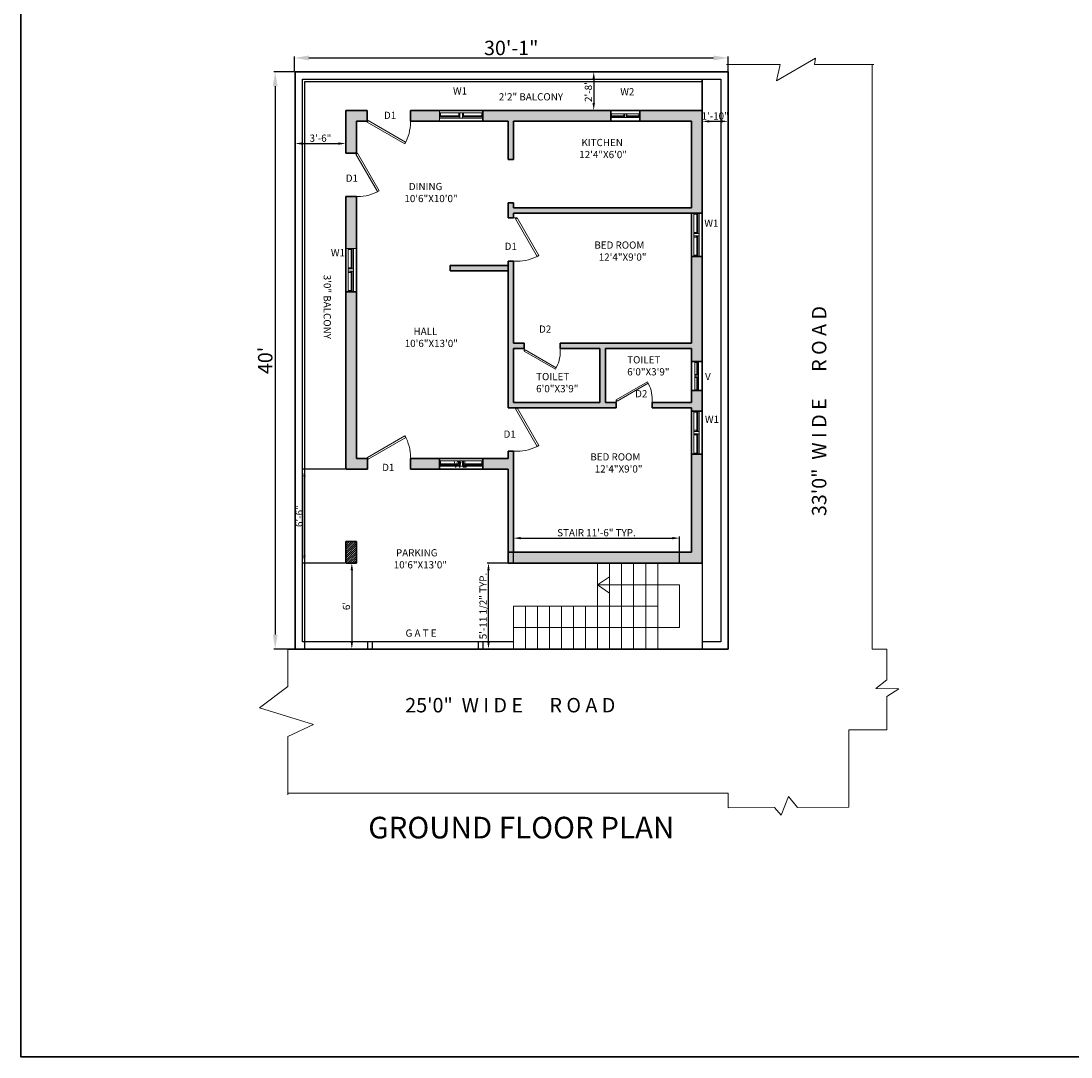
# Model space of a CAD drawing. Units: millimetres. Extents: x 50579 to 52843, y 62224 to 63803.
# Tile 1 of 5: x 50579 to 51453, y 62224 to 63086. Entities that reach past the tile are written whole.
import ezdxf

# ---------------------------------------------------------------- set-up
doc = ezdxf.new("R2010")
doc.units = ezdxf.units.MM
for name, color, linetype, lineweight in [('A-ANNO-DIMS', 2, 'Continuous', 18), ('A-ANNO-IDEN', 6, 'Continuous', 18), ('A-ANNO-TITL', 4, 'Continuous', 25), ('A-ANNO-TTLB', 7, 'Continuous', 35), ('A-AREA-IDEN', 6, 'Continuous', 18), ('A-COLS', 7, 'Continuous', 35), ('A-COLS-PATT', 8, 'Continuous', 13), ('A-FLOR-BALC', 7, 'Continuous', 25), ('A-FLOR-STRS', 7, 'Continuous', 18), ('A-GLAZ', 4, 'Continuous', 18), ('A-WALL', 7, 'Continuous', 35), ('A-WALL-PATT', 251, 'Continuous', 13), ('C-ANNO-TEXT', 4, 'Continuous', 18), ('C-PROP', 7, 'Continuous', 35), ('C-ROAD', 7, 'Continuous', 18), ('C-SITE-GATE', 7, 'Continuous', 25), ('C-SITE-WALL', 7, 'Continuous', 25), ('DOOR', 20, 'Continuous', 18)]:
    doc.layers.add(name, color=color, linetype=linetype, lineweight=lineweight)
doc.styles.get("Standard").update_dxf_attribs({"font": 'arial.ttf'})
doc.dimstyles.new('ISO-25', dxfattribs={"dimtxt": 6, "dimasz": 6, "dimexe": 1.25, "dimexo": 0.625, "dimtad": 1, "dimdec": 0, "dimlunit": 3, "dimtxsty": 'Standard', "dimcen": 2.5, "dimadec": 0, "dimazin": 0, "dimtfac": 1, "dimtdec": 0, "dimtmove": 0, "dimatfit": 3, "dimfxl": 1, "dimarcsym": 0})

# ---------------------------------------------------------------- blocks, each defined once
blk = doc.blocks.new('W1')
for p, q in [((50927.56, 62719.85), (50945.56, 62719.85)), ((50927.56, 62717.25), (50944.56, 62717.25)), ((50927.56, 62716.35), (50944.56, 62716.35)), ((50927.56, 62715.35), (50963.56, 62715.35)), ((50929.58, 62717.08), (50942.53, 62717.08)), ((50929.58, 62716.8), (50942.53, 62716.8)), ((50929.58, 62716.54), (50942.53, 62716.54)), ((50944.56, 62717.61), (50944.56, 62715.35)), ((50963.56, 62719.85), (50945.56, 62719.85)), ((50946.56, 62717.61), (50946.56, 62715.35)), ((50963.56, 62717.25), (50946.56, 62717.25)), ((50963.56, 62716.35), (50946.56, 62716.35)), ((50961.53, 62717.08), (50948.58, 62717.08)), ((50961.53, 62716.8), (50948.58, 62716.8)), ((50961.53, 62716.54), (50948.58, 62716.54))]:
    blk.add_line(p, q)
for points in [[(50927.56, 62712.85), (50927.56, 62721.85), (50963.56, 62721.85), (50963.56, 62712.85)], [(50927.56, 62719.85), (50928.5, 62719.85), (50928.5, 62717.61), (50927.56, 62717.61)], [(50928.59, 62717.25), (50929.58, 62717.25), (50929.58, 62716.35), (50928.59, 62716.35)], [(50943.52, 62717.25), (50942.53, 62717.25), (50942.53, 62716.35), (50943.52, 62716.35)], [(50944.56, 62719.85), (50943.61, 62719.85), (50943.61, 62717.61), (50944.56, 62717.61)], [(50946.56, 62719.85), (50947.5, 62719.85), (50947.5, 62717.61), (50946.56, 62717.61)], [(50947.59, 62717.25), (50948.58, 62717.25), (50948.58, 62716.35), (50947.59, 62716.35)], [(50962.52, 62717.25), (50961.53, 62717.25), (50961.53, 62716.35), (50962.52, 62716.35)], [(50963.56, 62719.85), (50962.61, 62719.85), (50962.61, 62717.61), (50963.56, 62717.61)]]:
    blk.add_lwpolyline(points, close=True)
blk = doc.blocks.new('*U3')
for p, q in [((0, 0), (0, -6)), ((40, 0), (40, -6))]:
    blk.add_line(p, q)
blk.add_lwpolyline([(0, 0), (34.64, 20), (35.52, 18.48), (0.87, -1.52)], close=True)
blk.add_arc((0, 0), 40, 0, 30)
blk = doc.blocks.new('*D5')
at = {"layer": 'A-ANNO-DIMS', "color": 0, "lineweight": -2, "transparency": 16777216}
for p, q in [((51052.14, 63043.35), (51057.07, 63043.35)), ((51055.82, 63037.35), (51055.82, 63017.35)), ((51052.14, 63011.35), (51057.07, 63011.35))]:
    blk.add_line(p, q, dxfattribs=at)
at = {"layer": 'A-ANNO-DIMS', "color": 0, "transparency": 16777216}
for points in [[(51054.82, 63037.35), (51056.82, 63037.35), (51055.82, 63043.35)], [(51054.82, 63017.35), (51056.82, 63017.35), (51055.82, 63011.35)]]:
    blk.add_solid(points, dxfattribs=at)
at = {"layer": 'Defpoints', "color": 0, "transparency": 16777216}
for p in [(51051.52, 63043.35), (51051.52, 63011.35), (51055.82, 63011.35)]:
    blk.add_point(p, dxfattribs=at)
at = {"layer": 'A-ANNO-DIMS', "color": 0, "transparency": 16777216, "insert": (51052.13, 63027.35), "char_height": 6, "attachment_point": 5, "rotation": 90}
blk.add_mtext('2\'-8"', dxfattribs=at)
blk = doc.blocks.new('*D6')
at = {"layer": 'A-ANNO-DIMS', "color": 0, "lineweight": -2, "transparency": 16777216}
for p, q in [((51146.02, 63010.73), (51146.02, 63000.95)), ((51167.52, 63010.73), (51167.52, 63000.95)), ((51161.52, 63002.2), (51152.02, 63002.2))]:
    blk.add_line(p, q, dxfattribs=at)
at = {"layer": 'A-ANNO-DIMS', "color": 0, "transparency": 16777216}
for points in [[(51152.02, 63003.2), (51152.02, 63001.2), (51146.02, 63002.2)], [(51161.52, 63003.2), (51161.52, 63001.2), (51167.52, 63002.2)]]:
    blk.add_solid(points, dxfattribs=at)
at = {"layer": 'Defpoints', "color": 0, "transparency": 16777216}
for p in [(51146.02, 63011.35), (51167.52, 63011.35), (51146.02, 63002.2)]:
    blk.add_point(p, dxfattribs=at)
at = {"layer": 'A-ANNO-DIMS', "color": 0, "transparency": 16777216, "insert": (51156.77, 63005.89), "char_height": 6, "attachment_point": 5}
blk.add_mtext('1\'-10"', dxfattribs=at)
blk = doc.blocks.new('*D7')
at = {"layer": 'A-ANNO-DIMS', "color": 0, "lineweight": -2, "transparency": 16777216}
for p, q in [((50807.52, 62977.26), (50807.52, 62984.99)), ((50813.52, 62983.74), (50843.52, 62983.74)), ((50849.52, 62977.26), (50849.52, 62984.99))]:
    blk.add_line(p, q, dxfattribs=at)
at = {"layer": 'A-ANNO-DIMS', "color": 0, "transparency": 16777216}
for points in [[(50813.52, 62984.74), (50813.52, 62982.74), (50807.52, 62983.74)], [(50843.52, 62984.74), (50843.52, 62982.74), (50849.52, 62983.74)]]:
    blk.add_solid(points, dxfattribs=at)
at = {"layer": 'Defpoints', "color": 0, "transparency": 16777216}
for p in [(50849.52, 62983.74), (50807.52, 62976.63), (50849.52, 62976.63)]:
    blk.add_point(p, dxfattribs=at)
at = {"layer": 'A-ANNO-DIMS', "color": 0, "transparency": 16777216, "insert": (50828.52, 62987.43), "char_height": 6, "attachment_point": 5}
blk.add_mtext('3\'-6"', dxfattribs=at)
blk = doc.blocks.new('*D8')
at = {"layer": 'A-ANNO-DIMS', "color": 0, "lineweight": -2, "transparency": 16777216}
for p, q in [((50806.89, 63043.35), (50789.64, 63043.35)), ((50790.89, 63031.35), (50790.89, 62575.35)), ((50806.89, 62563.35), (50789.64, 62563.35))]:
    blk.add_line(p, q, dxfattribs=at)
at = {"layer": 'A-ANNO-DIMS', "color": 0, "transparency": 16777216}
for points in [[(50788.89, 63031.35), (50792.89, 63031.35), (50790.89, 63043.35)], [(50788.89, 62575.35), (50792.89, 62575.35), (50790.89, 62563.35)]]:
    blk.add_solid(points, dxfattribs=at)
at = {"layer": 'Defpoints', "color": 0, "transparency": 16777216}
for p in [(50807.52, 63043.35), (50790.89, 62563.35), (50807.52, 62563.35)]:
    blk.add_point(p, dxfattribs=at)
at = {"layer": 'A-ANNO-DIMS', "color": 0, "transparency": 16777216, "insert": (50784.14, 62803.35), "char_height": 12, "attachment_point": 5, "rotation": 90}
blk.add_mtext("40'", dxfattribs=at)
blk = doc.blocks.new('*D9')
at = {"layer": 'A-ANNO-DIMS', "color": 0, "lineweight": -2, "transparency": 16777216}
for p, q in [((50806.89, 63043.98), (50806.89, 63056.19)), ((50818.89, 63054.94), (51155.52, 63054.94)), ((51167.52, 63043.98), (51167.52, 63056.19))]:
    blk.add_line(p, q, dxfattribs=at)
at = {"layer": 'A-ANNO-DIMS', "color": 0, "transparency": 16777216}
for points in [[(50818.89, 63056.94), (50818.89, 63052.94), (50806.89, 63054.94)], [(51155.52, 63056.94), (51155.52, 63052.94), (51167.52, 63054.94)]]:
    blk.add_solid(points, dxfattribs=at)
at = {"layer": 'Defpoints', "color": 0, "transparency": 16777216}
for p in [(51167.52, 63054.94), (50806.89, 63043.35), (51167.52, 63043.35)]:
    blk.add_point(p, dxfattribs=at)
at = {"layer": 'A-ANNO-DIMS', "color": 0, "transparency": 16777216, "insert": (50987.2, 63061.7), "char_height": 12, "attachment_point": 5}
blk.add_mtext('30\'-1"', dxfattribs=at)
blk = doc.blocks.new('*D10')
at = {"layer": 'A-ANNO-DIMS', "color": 0, "lineweight": -2, "transparency": 16777216}
for p, q in [((50854.64, 62634.85), (50855.88, 62634.85)), ((50854.63, 62628.85), (50854.63, 62569.35)), ((50854.64, 62563.35), (50855.88, 62563.35))]:
    blk.add_line(p, q, dxfattribs=at)
at = {"layer": 'A-ANNO-DIMS', "color": 0, "transparency": 16777216}
for points in [[(50853.63, 62628.85), (50855.63, 62628.85), (50854.63, 62634.85)], [(50853.63, 62569.35), (50855.63, 62569.35), (50854.63, 62563.35)]]:
    blk.add_solid(points, dxfattribs=at)
at = {"layer": 'Defpoints', "color": 0, "transparency": 16777216}
for p in [(50854.02, 62634.85), (50854.02, 62563.35), (50854.63, 62563.35)]:
    blk.add_point(p, dxfattribs=at)
at = {"layer": 'A-ANNO-DIMS', "color": 0, "transparency": 16777216, "insert": (50850.94, 62599.1), "char_height": 6, "attachment_point": 5, "rotation": 90}
blk.add_mtext("6'", dxfattribs=at)
blk = doc.blocks.new('WIN-W2-PLAN')
for p, q in [((0, 6.16), (12, 6.16)), ((0, 4.43), (11.33, 4.43)), ((0, 3.83), (11.33, 3.83)), ((0, 3.16), (24, 3.16)), ((1.35, 4.32), (9.98, 4.32)), ((1.35, 4.13), (9.98, 4.13)), ((1.35, 3.95), (9.98, 3.95)), ((11.33, 4.67), (11.33, 3.16)), ((24, 6.16), (12, 6.16)), ((12.67, 4.67), (12.67, 3.16)), ((24, 4.43), (12.67, 4.43)), ((24, 3.83), (12.67, 3.83)), ((22.65, 4.32), (14.02, 4.32)), ((22.65, 4.13), (14.02, 4.13)), ((22.65, 3.95), (14.02, 3.95))]:
    blk.add_line(p, q)
for points in [[(0, 0), (0, 9), (24, 9), (24, 0)], [(0, 6.16), (0.63, 6.16), (0.63, 4.67), (0, 4.67)], [(0.69, 4.43), (1.35, 4.43), (1.35, 3.83), (0.69, 3.83)], [(10.64, 4.43), (9.98, 4.43), (9.98, 3.83), (10.64, 3.83)], [(11.33, 6.16), (10.7, 6.16), (10.7, 4.67), (11.33, 4.67)], [(12.67, 6.16), (13.29, 6.16), (13.29, 4.67), (12.67, 4.67)], [(13.36, 4.43), (14.02, 4.43), (14.02, 3.83), (13.36, 3.83)], [(23.31, 4.43), (22.65, 4.43), (22.65, 3.83), (23.31, 3.83)], [(24, 6.16), (23.37, 6.16), (23.37, 4.67), (24, 4.67)]]:
    blk.add_lwpolyline(points, close=True)
blk = doc.blocks.new('VENT-V-PLAN')
for p, q in [((2.84, 24), (2.84, 12)), ((4.57, 24), (4.57, 12.67)), ((4.68, 22.65), (4.68, 14.02)), ((4.87, 22.65), (4.87, 14.02)), ((5.05, 22.65), (5.05, 14.02)), ((5.17, 24), (5.17, 12.67)), ((5.84, 24), (5.84, 0)), ((2.84, 0), (2.84, 12)), ((4.33, 12.67), (5.84, 12.67)), ((4.33, 11.33), (5.84, 11.33)), ((4.57, 0), (4.57, 11.33)), ((4.68, 1.35), (4.68, 9.98)), ((4.87, 1.35), (4.87, 9.98)), ((5.05, 1.35), (5.05, 9.98)), ((5.17, 0), (5.17, 11.33))]:
    blk.add_line(p, q)
for points in [[(9, 24), (0, 24), (0, 0), (9, 0)], [(2.84, 24), (2.84, 23.37), (4.33, 23.37), (4.33, 24)], [(4.57, 23.31), (4.57, 22.65), (5.17, 22.65), (5.17, 23.31)], [(2.84, 12.67), (2.84, 13.3), (4.33, 13.3), (4.33, 12.67)], [(2.84, 11.33), (2.84, 10.71), (4.33, 10.71), (4.33, 11.33)], [(4.57, 13.36), (4.57, 14.02), (5.17, 14.02), (5.17, 13.36)], [(4.57, 10.64), (4.57, 9.98), (5.17, 9.98), (5.17, 10.64)], [(2.84, 0), (2.84, 0.63), (4.33, 0.63), (4.33, 0)], [(4.57, 0.69), (4.57, 1.35), (5.17, 1.35), (5.17, 0.69)]]:
    blk.add_lwpolyline(points, close=True)
blk = doc.blocks.new('STAIR-RETURN-PLAN')
for p, q in [((70, 0), (70, 71.5)), ((80, 0), (80, 71.5)), ((90, 0), (90, 71.5)), ((100, 0), (100, 71.5)), ((110, 0), (110, 71.5)), ((120, 0), (120, 71.5)), ((70, 53.25), (80, 59.99)), ((138.14, 53.25), (70, 53.25)), ((70, 53.25), (80, 46.5)), ((138.14, 17.87), (138.14, 53.25)), ((0, 0), (0, 35.75)), ((120, 35.75), (0, 35.75)), ((10, 0), (10, 35.75)), ((20, 0), (20, 35.75)), ((30, 0), (30, 35.75)), ((40, 0), (40, 35.75)), ((50, 0), (50, 35.75)), ((60, 0), (60, 35.75)), ((0, 17.87), (138.14, 17.87))]:
    blk.add_line(p, q)
blk = doc.blocks.new('GATE-POST-PAIR')
for p, q in [((0, 6), (0, 0)), ((4, 6), (4, 0)), ((92.04, 6), (92.04, 0)), ((96.04, 6), (96.04, 0))]:
    blk.add_line(p, q)
blk = doc.blocks.new('*D33')
at = {"layer": 'A-ANNO-DIMS', "color": 0, "lineweight": -2, "transparency": 16777216}
for p, q in [((50989.02, 62635.48), (50989.02, 62656.82)), ((50995.02, 62655.57), (51121.16, 62655.57)), ((51127.16, 62635.48), (51127.16, 62656.82))]:
    blk.add_line(p, q, dxfattribs=at)
at = {"layer": 'A-ANNO-DIMS', "color": 0, "transparency": 16777216}
for points in [[(50995.02, 62656.57), (50995.02, 62654.57), (50989.02, 62655.57)], [(51121.16, 62656.57), (51121.16, 62654.57), (51127.16, 62655.57)]]:
    blk.add_solid(points, dxfattribs=at)
at = {"layer": 'Defpoints', "color": 0, "transparency": 16777216}
for p in [(51127.16, 62655.57), (50989.02, 62634.85), (51127.16, 62634.85)]:
    blk.add_point(p, dxfattribs=at)
at = {"layer": 'A-ANNO-DIMS', "color": 0, "transparency": 16777216, "insert": (51058.09, 62659.3), "char_height": 6, "attachment_point": 5}
blk.add_mtext('STAIR 11\'-6" TYP.', dxfattribs=at)
blk = doc.blocks.new('*D34')
at = {"layer": 'A-ANNO-DIMS', "color": 0, "lineweight": -2, "transparency": 16777216}
for p, q in [((50988.39, 62634.85), (50967.05, 62634.85)), ((50968.3, 62569.35), (50968.3, 62628.85)), ((50988.39, 62563.35), (50967.05, 62563.35))]:
    blk.add_line(p, q, dxfattribs=at)
at = {"layer": 'A-ANNO-DIMS', "color": 0, "transparency": 16777216}
for points in [[(50967.3, 62628.85), (50969.3, 62628.85), (50968.3, 62634.85)], [(50967.3, 62569.35), (50969.3, 62569.35), (50968.3, 62563.35)]]:
    blk.add_solid(points, dxfattribs=at)
at = {"layer": 'Defpoints', "color": 0, "transparency": 16777216}
for p in [(50968.3, 62634.85), (50989.02, 62634.85), (50989.02, 62563.35)]:
    blk.add_point(p, dxfattribs=at)
at = {"layer": 'A-ANNO-DIMS', "color": 0, "transparency": 16777216, "insert": (50964.57, 62599.1), "char_height": 6, "attachment_point": 5, "rotation": 90}
blk.add_mtext('5\'-11 1/2" TYP.', dxfattribs=at)
blk = doc.blocks.new('*D76')
at = {"layer": 'A-ANNO-DIMS', "color": 0, "lineweight": -2, "transparency": 16777216}
for p, q in [((50848.89, 62712.85), (50813.97, 62712.85)), ((50815.22, 62640.85), (50815.22, 62706.85)), ((50848.89, 62634.85), (50813.97, 62634.85))]:
    blk.add_line(p, q, dxfattribs=at)
at = {"layer": 'A-ANNO-DIMS', "color": 0, "transparency": 16777216}
for points in [[(50814.22, 62706.85), (50816.22, 62706.85), (50815.22, 62712.85)], [(50814.22, 62640.85), (50816.22, 62640.85), (50815.22, 62634.85)]]:
    blk.add_solid(points, dxfattribs=at)
at = {"layer": 'Defpoints', "color": 0, "transparency": 16777216}
for p in [(50815.22, 62712.85), (50849.52, 62712.85), (50849.52, 62634.85)]:
    blk.add_point(p, dxfattribs=at)
at = {"layer": 'A-ANNO-DIMS', "color": 0, "transparency": 16777216, "insert": (50811.53, 62673.85), "char_height": 6, "attachment_point": 5, "rotation": 90}
blk.add_mtext('6\'-6"', dxfattribs=at)

msp = doc.modelspace()

# ---------------------------------------------------------------- hatches: boundary and pattern name
at = {"layer": 'A-COLS-PATT'}
h = msp.add_hatch(dxfattribs=at)
h.set_pattern_fill('ANSI31', color=256, scale=0.4)
h.paths.add_polyline_path([(50858.52, 62643.85), (50858.52, 62652.85), (50849.52, 62652.85), (50849.52, 62634.85), (50858.52, 62634.85)])
at = {"layer": 'A-WALL-PATT'}
h = msp.add_hatch(color=256, dxfattribs=at)
h.dxf.hatch_style = 1
h.paths.add_polyline_path([(50858.52, 63002.35), (50867.4, 63002.35), (50867.4, 63006.85), (50867.4, 63011.35), (50849.52, 63011.35), (50849.52, 62975.7), (50858.52, 62975.7)])
h = msp.add_hatch(color=256, dxfattribs=at)
h.dxf.hatch_style = 1
h.paths.add_polyline_path([(50927.56, 63011.35), (50903.4, 63011.35), (50903.4, 63002.35), (50927.56, 63002.35)])
h = msp.add_hatch(color=256, dxfattribs=at)
h.dxf.hatch_style = 1
h.paths.add_polyline_path([(51070.05, 63011.35), (50963.56, 63011.35), (50963.56, 63002.35), (50984.52, 63002.35), (50984.52, 62970.35), (50989.02, 62970.35), (50989.02, 63002.35), (51070.05, 63002.35)])
h = msp.add_hatch(color=256, dxfattribs=at)
h.dxf.hatch_style = 1
h.paths.add_polyline_path([(51146.02, 63011.35), (51094.05, 63011.35), (51094.05, 63002.35), (51137.02, 63002.35), (51137.02, 62930.35), (50989.02, 62930.35), (50989.02, 62934.35), (50984.52, 62934.35), (50984.52, 62921.85), (50989.02, 62921.85), (50989.02, 62925.85), (51146.02, 62925.85)])
h = msp.add_hatch(color=256, dxfattribs=at)
h.dxf.hatch_style = 1
h.paths.add_polyline_path([(50858.52, 62939.7), (50854.02, 62939.7), (50849.52, 62939.7), (50849.52, 62896.5), (50858.52, 62896.5)])
h = msp.add_hatch(color=256, dxfattribs=at)
h.dxf.hatch_style = 1
h.paths.add_polyline_path([(51074.52, 62768.35), (51065.52, 62768.35), (51065.52, 62813.35), (51137.02, 62813.35), (51137.02, 62802.37), (51146.02, 62802.37), (51146.02, 62889.85), (51137.02, 62889.85), (51137.02, 62817.85), (51028.02, 62817.85), (51028.02, 62813.35), (51061.02, 62813.35), (51061.02, 62768.35), (50989.02, 62768.35), (50989.02, 62813.35), (50998.02, 62813.35), (50998.02, 62817.85), (50989.02, 62817.85), (50989.02, 62885.85), (50984.52, 62885.85), (50984.52, 62763.85), (51074.52, 62763.85)])
h = msp.add_hatch(color=256, dxfattribs=at)
h.dxf.hatch_style = 1
h.paths.add_polyline_path([(50984.52, 62882.35), (50936.52, 62882.35), (50936.52, 62877.85), (50984.52, 62877.85)])
h = msp.add_hatch(color=256, dxfattribs=at)
h.dxf.hatch_style = 1
h.paths.add_polyline_path([(50858.52, 62860.5), (50849.52, 62860.5), (50849.52, 62712.85), (50867.52, 62712.85), (50867.52, 62721.85), (50858.52, 62721.85)])
h = msp.add_hatch(color=256, dxfattribs=at)
h.dxf.hatch_style = 1
h.paths.add_polyline_path([(51146.02, 62778.37), (51137.02, 62778.37), (51137.02, 62768.35), (51104.52, 62768.35), (51104.52, 62766.1), (51104.52, 62763.85), (51137.02, 62763.85), (51137.02, 62761.3), (51146.02, 62761.3)])
h = msp.add_hatch(color=256, dxfattribs=at)
h.dxf.hatch_style = 1
h.paths.add_polyline_path([(50927.56, 62721.85), (50903.52, 62721.85), (50903.52, 62717.35), (50903.52, 62712.85), (50927.56, 62712.85)])
h = msp.add_hatch(color=256, dxfattribs=at)
h.dxf.hatch_style = 1
h.paths.add_polyline_path([(50989.02, 62727.85), (50984.52, 62727.85), (50984.52, 62721.85), (50963.56, 62721.85), (50963.56, 62712.85), (50984.52, 62712.85), (50984.52, 62643.85), (50989.02, 62643.85)])
h = msp.add_hatch(color=256, dxfattribs=at)
h.dxf.hatch_style = 1
h.paths.add_polyline_path([(51146.02, 62725.3), (51137.02, 62725.3), (51137.02, 62643.85), (50984.52, 62643.85), (50984.52, 62634.85), (51146.02, 62634.85)])

# ---------------------------------------------------------------- linework, layer by layer
at = {"layer": 'A-ANNO-TTLB'}
msp.add_lwpolyline([(50579.46, 63802.65), (52843.1, 63802.65), (52843.1, 62224.04), (50579.46, 62224.04)], close=True, dxfattribs=at)
at = {"layer": 'A-COLS'}
for p, q in [((50849.52, 62634.85), (50849.52, 62652.85)), ((50849.52, 62652.85), (50858.52, 62652.85)), ((50858.52, 62643.85), (50858.52, 62652.85)), ((50858.52, 62643.85), (50858.52, 62634.85)), ((50849.52, 62634.85), (50858.52, 62634.85))]:
    msp.add_line(p, q, dxfattribs=at)
at = {"layer": 'A-FLOR-BALC'}
for p, q in [((50815.52, 63035.35), (51146.02, 63035.35)), ((50815.52, 62563.35), (50815.52, 63035.35)), ((51146.02, 62634.85), (51146.02, 62563.35))]:
    msp.add_line(p, q, dxfattribs=at)
at = {"layer": 'A-WALL'}
for p, q in [((51146.02, 62634.85), (51146.02, 63037.35)), ((50849.52, 63011.35), (50867.4, 63011.35)), ((50849.52, 62975.7), (50849.52, 63011.35)), ((50867.4, 63002.35), (50867.4, 63011.35)), ((50903.4, 63002.35), (50903.4, 63011.35)), ((50903.4, 63011.35), (51146.02, 63011.35)), ((50963.56, 63011.35), (50963.56, 63002.35)), ((51070.05, 63011.35), (51070.05, 63002.35)), ((51094.05, 63011.35), (51094.05, 63002.35)), ((50858.52, 63002.35), (50867.4, 63002.35)), ((50858.52, 62975.7), (50858.52, 63002.35)), ((50903.4, 63002.35), (50984.52, 63002.35)), ((50984.52, 62970.35), (50984.52, 63002.35)), ((50989.02, 63002.35), (51137.02, 63002.35)), ((50989.02, 62970.35), (50989.02, 63002.35)), ((51137.02, 62930.35), (51137.02, 63002.35)), ((50849.52, 62975.7), (50858.52, 62975.7)), ((50984.52, 62970.35), (50989.02, 62970.35)), ((50849.52, 62939.7), (50858.52, 62939.7)), ((50849.52, 62712.85), (50849.52, 62939.7)), ((50858.52, 62877.85), (50858.52, 62939.7)), ((50984.52, 62934.35), (50989.02, 62934.35)), ((50984.52, 62921.85), (50984.52, 62934.35)), ((50989.02, 62930.35), (50989.02, 62934.35)), ((50989.02, 62930.35), (51137.02, 62930.35)), ((50984.52, 62921.85), (50989.02, 62921.85)), ((50989.02, 62925.85), (51146.02, 62925.85)), ((50989.02, 62921.85), (50989.02, 62925.85)), ((51137.02, 62817.85), (51137.02, 62925.85)), ((51137.02, 62889.85), (51146.02, 62889.85)), ((50858.52, 62721.85), (50858.52, 62877.85)), ((50936.52, 62882.35), (50984.52, 62882.35)), ((50936.52, 62877.85), (50936.52, 62882.35)), ((50936.52, 62877.85), (50984.52, 62877.85)), ((50984.52, 62885.85), (50989.02, 62885.85)), ((50984.52, 62763.85), (50984.52, 62885.85)), ((50989.02, 62817.85), (50989.02, 62885.85)), ((50849.52, 62860.5), (50858.52, 62860.5)), ((50989.02, 62817.85), (50998.02, 62817.85)), ((50998.02, 62813.35), (50998.02, 62817.85)), ((51028.02, 62813.35), (51028.02, 62817.85)), ((51028.02, 62817.85), (51137.02, 62817.85)), ((50989.02, 62813.35), (50998.02, 62813.35)), ((50989.02, 62768.35), (50989.02, 62813.35)), ((51028.02, 62813.35), (51061.02, 62813.35)), ((51061.02, 62768.35), (51061.02, 62813.35)), ((51065.52, 62768.35), (51065.52, 62813.35)), ((51065.52, 62813.35), (51137.02, 62813.35)), ((51137.02, 62768.35), (51137.02, 62813.35)), ((51137.02, 62802.37), (51146.02, 62802.37)), ((51137.02, 62778.37), (51146.02, 62778.37)), ((50984.52, 62763.85), (51074.52, 62763.85)), ((50989.02, 62768.35), (51061.02, 62768.35)), ((51065.52, 62768.35), (51074.52, 62768.35)), ((51074.52, 62768.35), (51074.52, 62763.85)), ((51104.52, 62768.35), (51104.52, 62763.85)), ((51104.52, 62768.35), (51137.02, 62768.35)), ((51104.52, 62763.85), (51137.02, 62763.85)), ((51137.02, 62643.85), (51137.02, 62763.85)), ((51137.02, 62761.3), (51146.02, 62761.3)), ((51137.02, 62761.3), (51146.02, 62761.3)), ((50858.52, 62721.85), (50867.52, 62721.85)), ((50867.52, 62721.85), (50867.52, 62712.85)), ((50903.52, 62721.85), (50903.52, 62712.85)), ((50903.52, 62721.85), (50984.52, 62721.85)), ((50927.56, 62721.85), (50927.56, 62712.85)), ((50963.56, 62721.85), (50963.56, 62712.85)), ((50984.52, 62721.85), (50984.52, 62727.85)), ((50984.52, 62727.85), (50989.02, 62727.85)), ((50989.02, 62643.85), (50989.02, 62727.85)), ((51137.02, 62725.3), (51146.02, 62725.3)), ((50849.52, 62712.85), (50867.52, 62712.85)), ((50903.52, 62712.85), (50984.52, 62712.85)), ((50984.52, 62634.85), (50984.52, 62712.85)), ((50984.52, 62643.85), (51137.02, 62643.85)), ((50984.52, 62634.85), (51146.02, 62634.85))]:
    msp.add_line(p, q, dxfattribs=at)
at = {"layer": 'C-PROP'}
for p, q in [((50807.52, 63043.35), (51167.52, 63043.35)), ((50807.52, 62563.35), (50807.52, 63043.35)), ((51167.52, 63043.35), (51167.52, 62563.35)), ((51167.52, 62563.35), (50801.52, 62563.35))]:
    msp.add_line(p, q, dxfattribs=at)
at = {"layer": 'C-ROAD'}
for p, q in [((51167.52, 63043.35), (51167.52, 63049.35)), ((51287.52, 63049.35), (51287.52, 62563.35)), ((51287.52, 62563.35), (51299.52, 62563.35)), ((51299.52, 62496.1), (51268.03, 62496.1)), ((51268.03, 62496.1), (51268.03, 62431.93)), ((51167.52, 62443.35), (50801.52, 62443.35)), ((51167.52, 62443.35), (51167.52, 62431.35))]:
    msp.add_line(p, q, dxfattribs=at)
for points in [[(51166.27, 63049.35), (51210.88, 63049.35), (51207.92, 63035.88), (51240.29, 63054.68), (51239.47, 63049.35), (51288.77, 63049.35)], [(50801.52, 62563.35), (50801.52, 62532.29), (50777.75, 62514.45), (50822.6, 62500.69), (50801.52, 62490.48), (50801.52, 62442.1)], [(51299.52, 62563.35), (51299.52, 62537.62), (51290.37, 62530.48), (51309.6, 62530.23), (51299.52, 62523.87), (51299.52, 62496.1)], [(51167.52, 62431.35), (51206.09, 62431.58), (51211.79, 62425.16), (51217.9, 62440.74), (51225.26, 62431.66), (51268.03, 62431.93)]]:
    msp.add_lwpolyline(points, dxfattribs=at)
at = {"layer": 'C-SITE-WALL'}
for p, q in [((50813.52, 63037.35), (51161.52, 63037.35)), ((50813.52, 62569.35), (50813.52, 63037.35)), ((51161.52, 63037.35), (51161.52, 62569.35)), ((50989.02, 62569.35), (50813.52, 62569.35)), ((51161.52, 62569.35), (51146.02, 62569.35))]:
    msp.add_line(p, q, dxfattribs=at)

# ---------------------------------------------------------------- block references
at = {"layer": 'A-FLOR-STRS'}
msp.add_blockref('STAIR-RETURN-PLAN', (50989.02, 62563.35), dxfattribs=at)
at = {"layer": 'A-GLAZ'}
for name, p in [('W1', (0, 289.5)), ('WIN-W2-PLAN', (51070.05, 63002.35)), ('VENT-V-PLAN', (51137.02, 62778.37)), ('W1', (0, 0))]:
    msp.add_blockref(name, p, dxfattribs=at)
at = {"layer": 'A-GLAZ', "rotation": 90}
for p in [(113858.87, 11962.3), (113571.37, 11932.94), (113858.87, 11797.74)]:
    msp.add_blockref('W1', p, dxfattribs=at)
at = {"layer": 'C-SITE-GATE'}
msp.add_blockref('GATE-POST-PAIR', (50867.52, 62563.35), dxfattribs=at)
at = {"layer": 'DOOR'}
for p, xscale, yscale, zscale, rotation in [((50867.4, 63001.45), -0.9, 0.9, 0.9, 180), ((50859.42, 62975.7), 0.9, 0.9, 0.9, 270), ((50992.17, 62921.85), 0.9, 0.9, 0.9, 270), ((50998.02, 62811.1), -0.75, 0.75, 0.75, 180), ((50992.17, 62763.85), 0.9, 0.9, 0.9, 270)]:
    msp.add_blockref('*U3', p, dxfattribs=dict(at, xscale=xscale, yscale=yscale, zscale=zscale, rotation=rotation))
for p, xscale, yscale, zscale in [((51074.52, 62770.6), 0.7499999999998483, 0.7499999999998483, 0.7499999999998483), ((50867.52, 62722.75), 0.9, 0.9, 0.9)]:
    msp.add_blockref('*U3', p, dxfattribs=dict(at, xscale=xscale, yscale=yscale, zscale=zscale))

# ---------------------------------------------------------------- texts
at = {"layer": 'A-ANNO-IDEN', "char_height": 6, "attachment_point": 1}
for s, insert in [('  W1', (50938.77, 63030.53)), ('  W2', (51077.87, 63029.83)), ('  D1', (50877.66, 63010.21)), ('  D1', (50845.93, 62957.95)), ('  W1', (51147.8, 62920.52)), ('  W1', (50837.19, 62895.97)), ('  D1', (50978.02, 62901.25)), ('  D2', (51006.67, 62832.42)), ('  V', (51144.73, 62792.98)), ('  D2', (51086.58, 62778.71)), ('  W1', (51148.3, 62757.41)), ('  D1', (50977.16, 62745.08)), ('  W1', (50939.03, 62720.29)), ('  D1', (50876.19, 62717.39))]:
    msp.add_mtext_dynamic_manual_height_columns(s, width=13.8936, gutter_width=12.5, heights=[0], dxfattribs=dict(at, insert=insert))
at = {"layer": 'A-ANNO-TITL', "insert": (50857.28, 62423.82), "char_height": 18, "attachment_point": 1}
msp.add_mtext_dynamic_manual_height_columns('  GROUND FLOOR PLAN', width=341.9217, gutter_width=12.5, heights=[0], dxfattribs=at)
at = {"layer": 'A-AREA-IDEN', "char_height": 6, "attachment_point": 1}
for s, width, insert in [('  2\'2" BALCONY', 88.9546, (50973.2, 63025.62)), ('  KITCHEN\\P 12\'4"X6\'0"', 46.1696, (51041.91, 62987.6)), ('  DINING\\P10\'6"X10\'0"', 46.1696, (50898.35, 62951.01)), ('  BED ROOM \\P    12\'4"X9\'0"', 60.368, (51052.63, 62902.32)), ('    HALL\\P10\'6"X13\'0"', 46.1696, (50898.58, 62830.5)), ('  TOILET\\P  6\'0"X3\'9"', 46.1696, (51079.98, 62806.89)), ('  TOILET\\P  6\'0"X3\'9"', 46.1696, (51004.23, 62792.9)), ('  BED ROOM \\P    12\'4"X9\'0"', 60.368, (51049.3, 62726.14)), (' PARKING\\P10\'6"X13\'0"', 46.1696, (50889.48, 62646.38))]:
    msp.add_mtext_dynamic_manual_height_columns(s, width=width, gutter_width=12.5, heights=[0], dxfattribs=dict(at, insert=insert))
at = {"layer": 'A-AREA-IDEN', "insert": (50837.19, 62878.29), "char_height": 6, "attachment_point": 1, "rotation": 270}
msp.add_mtext_dynamic_manual_height_columns('  3\'0" BALCONY', width=88.9546, gutter_width=12.5, heights=[0], dxfattribs=at)
at = {"layer": 'C-ANNO-TEXT', "insert": (51237.29, 62666.56), "char_height": 12, "attachment_point": 1, "rotation": 90}
msp.add_mtext_dynamic_manual_height_columns('  33\'0"  W I D E      R O A D', width=227.2367, gutter_width=12.5, heights=[0], dxfattribs=at)
at = {"layer": 'C-ANNO-TEXT', "attachment_point": 1}
for s, width, insert, char_height in [('  G A T E', 46.1696, (50895.62, 62579.59), 6), ('  25\'0"  W I D E      R O A D', 227.2367, (50891.7, 62522.64), 12)]:
    msp.add_mtext_dynamic_manual_height_columns(s, width=width, gutter_width=12.5, heights=[0], dxfattribs=dict(at, insert=insert, char_height=char_height))

# ---------------------------------------------------------------- dimensions: what is measured, and where the dimension line sits
at = {"layer": 'A-ANNO-DIMS'}
for base, p1, p2, override, picture, middle in [((51167.52, 63054.94), (50806.89, 63043.35), (51167.52, 63043.35), {"dimtxt": 12, "dimasz": 12, "dimclrd": 0, "dimclre": 0, "dimclrt": 0}, '*D9', (50987.2, 63061.7)), ((51146.01677688, 63002.19843281), (51167.51677688, 63011.35192686), (51146.01677688, 63011.35192686), {"dimclrd": 0, "dimclre": 0, "dimclrt": 0}, '*D6', (51156.76677688, 63005.88687074)), ((50849.52, 62983.74), (50807.52, 62976.63), (50849.52, 62976.63), {"dimclrd": 0, "dimclre": 0, "dimclrt": 0}, '*D7', (50828.52, 62987.43))]:
    dim = msp.add_linear_dim(base=base, p1=p1, p2=p2, dimstyle='ISO-25', override=override, dxfattribs=at)
    dim.commit()
    dim.dimension.update_dxf_attribs({"geometry": picture, "text_midpoint": middle})
for base, p1, p2, override, picture, middle in [((50790.89, 62563.35), (50807.52, 63043.35), (50807.52, 62563.35), {"dimtxt": 12, "dimasz": 12, "dimclrd": 0, "dimclre": 0, "dimclrt": 0}, '*D8', (50784.14, 62803.35)), ((51055.82, 63011.35), (51051.52, 63043.35), (51051.52, 63011.35), {"dimclrd": 0, "dimclre": 0, "dimclrt": 0}, '*D5', (51052.13, 63027.35)), ((50815.22, 62712.85), (50849.52, 62634.85), (50849.52, 62712.85), {"dimdec": 1, "dimlfac": 1, "dimrnd": 0, "dimzin": 1, "dimdsep": 46, "dimlunit": 4, "dimfrac": 2}, '*D76', (50811.53, 62673.85)), ((50854.63084235, 62563.35192686), (50854.01677688, 62634.85192686), (50854.01677688, 62563.35192686), {"dimclrd": 0, "dimclre": 0, "dimclrt": 0}, '*D10', (50850.94240442, 62599.10192686))]:
    dim = msp.add_linear_dim(base=base, p1=p1, p2=p2, angle=90, dimstyle='ISO-25', override=override, dxfattribs=at)
    dim.commit()
    dim.dimension.update_dxf_attribs({"geometry": picture, "text_midpoint": middle})
dim = msp.add_linear_dim(base=(51127.16, 62655.57), p1=(50989.02, 62634.85), p2=(51127.16, 62634.85), text='STAIR <> TYP.', dimstyle='ISO-25', override={"dimdec": 1, "dimlfac": 1, "dimrnd": 0, "dimzin": 1, "dimdsep": 46, "dimlunit": 4, "dimfrac": 2}, dxfattribs=at)
dim.commit()
dim.dimension.update_dxf_attribs({"geometry": '*D33', "text_midpoint": (51058.09, 62659.3)})
dim = msp.add_linear_dim(base=(50968.3, 62634.85), p1=(50989.02, 62563.35), p2=(50989.02, 62634.85), angle=90, text='<> TYP.', dimstyle='ISO-25', override={"dimdec": 1, "dimlfac": 1, "dimrnd": 0, "dimzin": 1, "dimdsep": 46, "dimlunit": 4, "dimfrac": 2}, dxfattribs=at)
dim.commit()
dim.dimension.update_dxf_attribs({"geometry": '*D34', "text_midpoint": (50964.57, 62599.1)})

doc.saveas('drawing.dxf')
